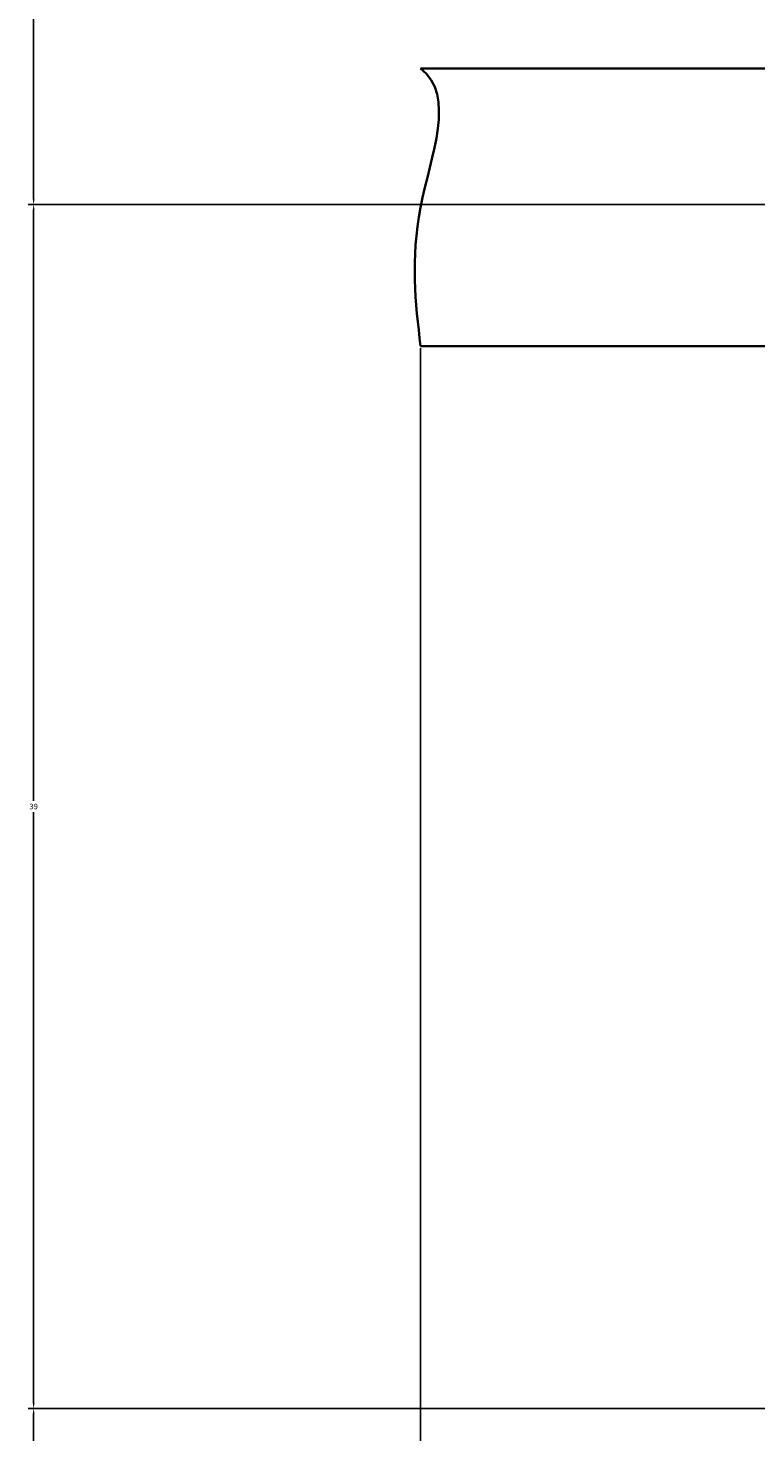
# Model space of a CAD drawing. Units: inches. Extents: x 2812 to 3051, y 1398 to 1659.
# Tile 45 of 65: x 2812 to 2835, y 1559 to 1605. Entities that reach past the tile are written whole.
import ezdxf

# ---------------------------------------------------------------- set-up
doc = ezdxf.new("R2010")
doc.units = ezdxf.units.IN
doc.layers.add('A-ANNO-DIMS', color=2, linetype='Continuous', lineweight=18)
doc.layers.add('P-SANR-PIPE', color=4, linetype='Continuous', lineweight=35)
doc.styles.get("Standard").update_dxf_attribs({"font": 'arial.ttf'})
doc.dimstyles.get("Standard").update_dxf_attribs({"dimtxt": 0.18, "dimasz": 0.18, "dimexe": 0.18, "dimexo": 0.0625, "dimgap": 0.09, "dimtad": 0, "dimtih": 1, "dimtoh": 1, "dimdec": 4, "dimzin": 0, "dimdsep": 46, "dimtxsty": 'Standard', "dimcen": 0.09, "dimadec": 0, "dimazin": 0, "dimtfac": 1, "dimtdec": 4, "dimtofl": 0, "dimtmove": 0, "dimatfit": 3, "dimfxl": 1, "dimtolj": 1, "dimtzin": 0, "dimarcsym": 0})

# ---------------------------------------------------------------- blocks, each defined once
blk = doc.blocks.new('PIPE-BREAK')
for p, q in [((27.315, 9), (0.19, 9)), ((0.19, 0), (27.315, 0))]:
    blk.add_line(p, q)
blk.add_open_spline([(0.19, 0), (0.025, 1.41), (-0.305, 4.231), (1.347, 8.126), (0.19, 9)], degree=3)
blk = doc.blocks.new('*D27')
at = {"layer": 'A-ANNO-DIMS', "color": 0, "lineweight": -2, "transparency": 16777216}
for p, q in [((2824.521, 1594.167), (2824.521, 1397.505)), ((2835.385, 1550.757), (2835.385, 1397.505)), ((2824.701, 1397.685), (2829.498, 1397.685)), ((2835.205, 1397.685), (2830.408, 1397.685))]:
    blk.add_line(p, q, dxfattribs=at)
at = {"layer": 'A-ANNO-DIMS', "color": 0, "transparency": 16777216}
for points in [[(2824.701, 1397.715), (2824.701, 1397.655), (2824.521, 1397.685)], [(2835.205, 1397.715), (2835.205, 1397.655), (2835.385, 1397.685)]]:
    blk.add_solid(points, dxfattribs=at)
at = {"layer": 'Defpoints', "color": 0, "transparency": 16777216}
for p in [(2824.521, 1594.23), (2835.385, 1550.82), (2835.385, 1397.685)]:
    blk.add_point(p, dxfattribs=at)
at = {"layer": 'A-ANNO-DIMS', "color": 0, "transparency": 16777216, "insert": (2829.953, 1397.685), "char_height": 0.18, "attachment_point": 5}
blk.add_mtext('\\A1;10.863', dxfattribs=at)
blk = doc.blocks.new('*D36')
at = {"layer": 'A-ANNO-DIMS', "color": 0, "lineweight": -2, "transparency": 16777216}
for p, q in [((2844.322, 1559.82), (2811.806, 1559.82)), ((2811.986, 1559.64), (2811.986, 1555.502)), ((2811.986, 1551), (2811.986, 1555.138)), ((2835.322, 1550.82), (2811.806, 1550.82))]:
    blk.add_line(p, q, dxfattribs=at)
at = {"layer": 'A-ANNO-DIMS', "color": 0, "transparency": 16777216}
for points in [[(2811.956, 1559.64), (2812.016, 1559.64), (2811.986, 1559.82)], [(2811.956, 1551), (2812.016, 1551), (2811.986, 1550.82)]]:
    blk.add_solid(points, dxfattribs=at)
at = {"layer": 'Defpoints', "color": 0, "transparency": 16777216}
for p in [(2811.986, 1559.82), (2844.385, 1559.82), (2835.385, 1550.82)]:
    blk.add_point(p, dxfattribs=at)
at = {"layer": 'A-ANNO-DIMS', "color": 0, "transparency": 16777216, "insert": (2811.986, 1555.32), "char_height": 0.18, "attachment_point": 5}
blk.add_mtext('\\A1;9', dxfattribs=at)
blk = doc.blocks.new('*D37')
at = {"layer": 'A-ANNO-DIMS', "color": 0, "lineweight": -2, "transparency": 16777216}
for p, q in [((2910.679, 1598.82), (2811.806, 1598.82)), ((2811.986, 1598.64), (2811.986, 1579.502)), ((2811.986, 1560), (2811.986, 1579.138)), ((2883.322, 1559.82), (2811.806, 1559.82))]:
    blk.add_line(p, q, dxfattribs=at)
at = {"layer": 'A-ANNO-DIMS', "color": 0, "transparency": 16777216}
for points in [[(2811.956, 1598.64), (2812.016, 1598.64), (2811.986, 1598.82)], [(2811.956, 1560), (2812.016, 1560), (2811.986, 1559.82)]]:
    blk.add_solid(points, dxfattribs=at)
at = {"layer": 'Defpoints', "color": 0, "transparency": 16777216}
for p in [(2811.986, 1598.82), (2910.742, 1598.82), (2883.385, 1559.82)]:
    blk.add_point(p, dxfattribs=at)
at = {"layer": 'A-ANNO-DIMS', "color": 0, "transparency": 16777216, "insert": (2811.986, 1579.32), "char_height": 0.18, "attachment_point": 5}
blk.add_mtext('\\A1;39', dxfattribs=at)
blk = doc.blocks.new('*D38')
at = {"layer": 'A-ANNO-DIMS', "color": 0, "lineweight": -2, "transparency": 16777216}
for p, q in [((2896.322, 1625.82), (2811.806, 1625.82)), ((2811.986, 1625.64), (2811.986, 1612.5)), ((2811.986, 1599), (2811.986, 1612.14)), ((2910.679, 1598.82), (2811.806, 1598.82))]:
    blk.add_line(p, q, dxfattribs=at)
at = {"layer": 'A-ANNO-DIMS', "color": 0, "transparency": 16777216}
for points in [[(2811.956, 1625.64), (2812.016, 1625.64), (2811.986, 1625.82)], [(2811.956, 1599), (2812.016, 1599), (2811.986, 1598.82)]]:
    blk.add_solid(points, dxfattribs=at)
at = {"layer": 'Defpoints', "color": 0, "transparency": 16777216}
for p in [(2811.986, 1625.82), (2896.385, 1625.82), (2910.742, 1598.82)]:
    blk.add_point(p, dxfattribs=at)
at = {"layer": 'A-ANNO-DIMS', "color": 0, "transparency": 16777216, "insert": (2811.986, 1612.32), "char_height": 0.18, "attachment_point": 5}
blk.add_mtext('\\A1;27', dxfattribs=at)

msp = doc.modelspace()

# ---------------------------------------------------------------- block references
at = {"layer": 'P-SANR-PIPE'}
msp.add_blockref('PIPE-BREAK', (2824.331, 1594.23), dxfattribs=at)

# ---------------------------------------------------------------- dimensions: what is measured, and where the dimension line sits
at = {"layer": 'A-ANNO-DIMS'}
for base, p1, p2, picture, middle in [((2811.9855, 1625.82), (2910.7415, 1598.82), (2896.3849, 1625.82), '*D38', (2811.9855, 1612.32)), ((2811.9855, 1598.82), (2883.3849, 1559.82), (2910.7415, 1598.82), '*D37', (2811.9855, 1579.32)), ((2811.9855, 1559.82), (2835.3849, 1550.82), (2844.3849, 1559.82), '*D36', (2811.9855, 1555.32))]:
    dim = msp.add_linear_dim(base=base, p1=p1, p2=p2, angle=90, dimstyle='Standard', override={"dimdec": 0, "dimlfac": 1, "dimrnd": 0, "dimzin": 0, "dimdsep": 46, "dimlunit": 2}, dxfattribs=at)
    dim.commit()
    dim.dimension.update_dxf_attribs({"geometry": picture, "text_midpoint": middle})
dim = msp.add_linear_dim(base=(2835.384907, 1397.685398), p1=(2824.521409, 1594.229631), p2=(2835.384907, 1550.819971), dimstyle='Standard', override={"dimdec": 3, "dimlfac": 1, "dimrnd": 0, "dimzin": 0, "dimdsep": 46, "dimlunit": 2}, dxfattribs=at)
dim.commit()
dim.dimension.update_dxf_attribs({"geometry": '*D27', "text_midpoint": (2829.953158, 1397.685398)})

doc.saveas('drawing.dxf')
